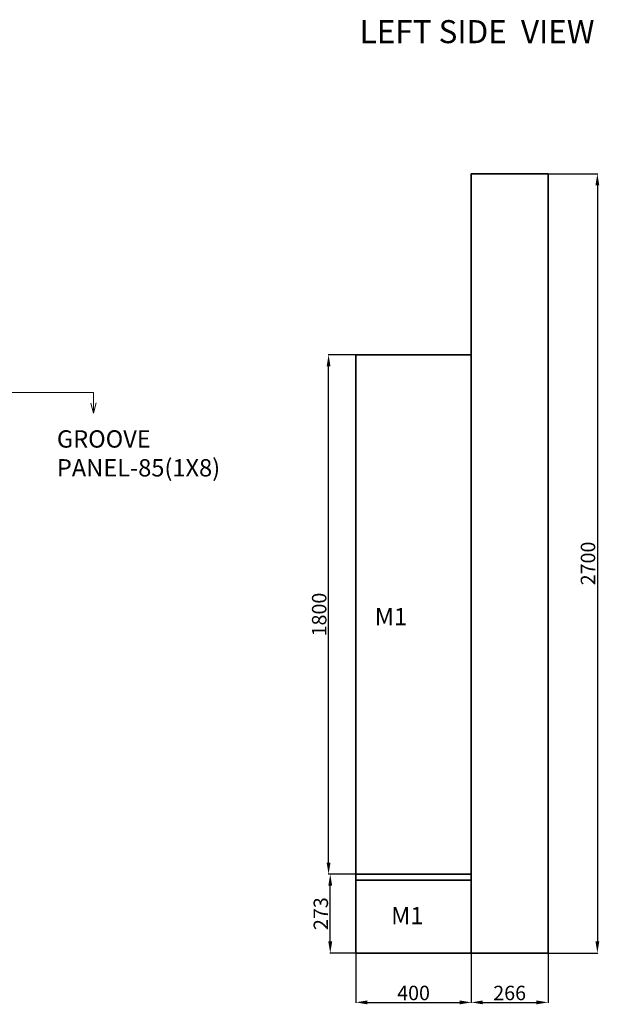
# Model space of a CAD drawing. Units: millimetres. Extents: x 11439 to 24661, y -4767 to -6.
# Tile 5 of 5: x 22652 to 24661, y -4215 to -803. Entities that reach past the tile are written whole.
import ezdxf

# ---------------------------------------------------------------- set-up
doc = ezdxf.new("R2010")
doc.units = ezdxf.units.MM
for name, color, linetype, lineweight in [('A-ANNO-DIMS', 2, 'Continuous', 18), ('A-ANNO-TEXT', 3, 'Continuous', 18), ('A-FURN', 7, 'Continuous', 35)]:
    doc.layers.add(name, color=color, linetype=linetype, lineweight=lineweight)
doc.styles.get("Standard").update_dxf_attribs({"font": 'arial.ttf'})
doc.dimstyles.new('ISO-25', dxfattribs={"dimtxt": 50, "dimasz": 40, "dimexe": 1.25, "dimexo": 0.625, "dimtad": 1, "dimtxsty": 'Standard', "dimcen": 2.5, "dimadec": 0, "dimazin": 0, "dimtfac": 1, "dimtmove": 0, "dimatfit": 3, "dimfxl": 1, "dimarcsym": 0})

# ---------------------------------------------------------------- blocks, each defined once
blk = doc.blocks.new('*D43')
at = {"layer": 'A-ANNO-DIMS', "color": 0, "lineweight": -2, "transparency": 16777216}
for p, q in [((23816.4, -3764.7), (23727.1, -3764.7)), ((23728.3, -3997.7), (23728.3, -3804.7)), ((23816.4, -4037.7), (23727.1, -4037.7))]:
    blk.add_line(p, q, dxfattribs=at)
at = {"layer": 'A-ANNO-DIMS', "color": 0, "transparency": 16777216}
for points in [[(23721.6, -3804.7), (23735, -3804.7), (23728.3, -3764.7)], [(23721.6, -3997.7), (23735, -3997.7), (23728.3, -4037.7)]]:
    blk.add_solid(points, dxfattribs=at)
at = {"layer": 'Defpoints', "color": 0, "transparency": 16777216}
for p in [(23728.3, -3764.7), (23817, -3764.7), (23817, -4037.7)]:
    blk.add_point(p, dxfattribs=at)
at = {"layer": 'A-ANNO-DIMS', "color": 0, "transparency": 16777216, "insert": (23702.1, -3901.2), "char_height": 50, "attachment_point": 5, "rotation": 90}
blk.add_mtext('273', dxfattribs=at)
blk = doc.blocks.new('*D44')
at = {"layer": 'A-ANNO-DIMS', "color": 0, "lineweight": -2, "transparency": 16777216}
for p, q in [((23816.4, -1964.7), (23721.3, -1964.7)), ((23722.5, -3724.7), (23722.5, -2004.7)), ((23816.4, -3764.7), (23721.3, -3764.7))]:
    blk.add_line(p, q, dxfattribs=at)
at = {"layer": 'A-ANNO-DIMS', "color": 0, "transparency": 16777216}
for points in [[(23715.8, -2004.7), (23729.2, -2004.7), (23722.5, -1964.7)], [(23715.8, -3724.7), (23729.2, -3724.7), (23722.5, -3764.7)]]:
    blk.add_solid(points, dxfattribs=at)
at = {"layer": 'Defpoints', "color": 0, "transparency": 16777216}
for p in [(23722.5, -1964.7), (23817, -1964.7), (23817, -3764.7)]:
    blk.add_point(p, dxfattribs=at)
at = {"layer": 'A-ANNO-DIMS', "color": 0, "transparency": 16777216, "insert": (23696.4, -2864.7), "char_height": 50, "attachment_point": 5, "rotation": 90}
blk.add_mtext('1800', dxfattribs=at)
blk = doc.blocks.new('*D54')
at = {"layer": 'A-ANNO-DIMS', "color": 0, "lineweight": -2, "transparency": 16777216}
for p, q in [((23817, -4038.3), (23817, -4209.9)), ((24217, -4038.3), (24217, -4209.9)), ((23857, -4208.7), (24177, -4208.7))]:
    blk.add_line(p, q, dxfattribs=at)
at = {"layer": 'A-ANNO-DIMS', "color": 0, "transparency": 16777216}
for points in [[(23857, -4202), (23857, -4215.4), (23817, -4208.7)], [(24177, -4202), (24177, -4215.4), (24217, -4208.7)]]:
    blk.add_solid(points, dxfattribs=at)
at = {"layer": 'Defpoints', "color": 0, "transparency": 16777216}
for p in [(23817, -4037.7), (24217, -4037.7), (24217, -4208.7)]:
    blk.add_point(p, dxfattribs=at)
at = {"layer": 'A-ANNO-DIMS', "color": 0, "transparency": 16777216, "insert": (24017, -4182.5), "char_height": 50, "attachment_point": 5}
blk.add_mtext('400', dxfattribs=at)
blk = doc.blocks.new('*D55')
at = {"layer": 'A-ANNO-DIMS', "color": 0, "lineweight": -2, "transparency": 16777216}
for p, q in [((24217, -4038.3), (24217, -4209.9)), ((24483, -4038.3), (24483, -4209.9)), ((24257, -4208.7), (24443, -4208.7))]:
    blk.add_line(p, q, dxfattribs=at)
at = {"layer": 'A-ANNO-DIMS', "color": 0, "transparency": 16777216}
for points in [[(24257, -4202), (24257, -4215.4), (24217, -4208.7)], [(24443, -4202), (24443, -4215.4), (24483, -4208.7)]]:
    blk.add_solid(points, dxfattribs=at)
at = {"layer": 'Defpoints', "color": 0, "transparency": 16777216}
for p in [(24217, -4037.7), (24483, -4037.7), (24483, -4208.7)]:
    blk.add_point(p, dxfattribs=at)
at = {"layer": 'A-ANNO-DIMS', "color": 0, "transparency": 16777216, "insert": (24350, -4182.5), "char_height": 50, "attachment_point": 5}
blk.add_mtext('266', dxfattribs=at)
blk = doc.blocks.new('*D56')
at = {"layer": 'A-ANNO-DIMS', "color": 0, "lineweight": -2, "transparency": 16777216}
for p, q in [((24483.6, -1337.7), (24655.3, -1337.7)), ((24654, -1377.7), (24654, -3997.7)), ((24483.6, -4037.7), (24655.3, -4037.7))]:
    blk.add_line(p, q, dxfattribs=at)
at = {"layer": 'A-ANNO-DIMS', "color": 0, "transparency": 16777216}
for points in [[(24647.3, -1377.7), (24660.7, -1377.7), (24654, -1337.7)], [(24647.3, -3997.7), (24660.7, -3997.7), (24654, -4037.7)]]:
    blk.add_solid(points, dxfattribs=at)
at = {"layer": 'Defpoints', "color": 0, "transparency": 16777216}
for p in [(24483, -1337.7), (24483, -4037.7), (24654, -4037.7)]:
    blk.add_point(p, dxfattribs=at)
at = {"layer": 'A-ANNO-DIMS', "color": 0, "transparency": 16777216, "insert": (24627.9, -2687.7), "char_height": 50, "attachment_point": 5, "rotation": 90}
blk.add_mtext('2700', dxfattribs=at)

msp = doc.modelspace()

# ---------------------------------------------------------------- linework, layer by layer
at = {"layer": 'A-ANNO-TEXT'}
for p, q in [((21560.761, -2095.642), (22907.534, -2095.642)), ((22907.534, -2095.642), (22907.534, -2166.511)), ((22907.534, -2166.511), (22898.054, -2132.022)), ((22907.534, -2166.511), (22917.263, -2131.108))]:
    msp.add_line(p, q, dxfattribs=at)
at = {"layer": 'A-FURN'}
for p, q in [((24217.007, -1337.684), (24483.007, -1337.684)), ((24217.007, -1337.684), (24217.007, -4037.684)), ((24483.007, -1337.684), (24483.007, -4037.684)), ((23817.007, -4037.684), (23817.007, -1964.684)), ((23817.007, -1964.684), (24217.007, -1964.684)), ((23817.007, -3764.684), (24217.007, -3764.684)), ((23817.007, -3784.684), (24217.007, -3784.684)), ((23817.007, -4037.684), (24483.007, -4037.684))]:
    msp.add_line(p, q, dxfattribs=at)

# ---------------------------------------------------------------- texts
at = {"layer": 'A-ANNO-TEXT', "attachment_point": 1}
for s, insert, char_height in [('LEFT SIDE  VIEW', (23830.171, -804.835), 80), ('GROOVE \\PPANEL-85(1X8)', (22780.973, -2226.26), 60), ('\\P    M1', (23809.23, -2741.895), 60), ('\\P    M1', (23865.925, -3777.968), 60)]:
    msp.add_mtext_dynamic_manual_height_columns(s, width=1074.7282, gutter_width=12.5, heights=[0], dxfattribs=dict(at, insert=insert, char_height=char_height))

# ---------------------------------------------------------------- dimensions: what is measured, and where the dimension line sits
at = {"layer": 'A-ANNO-DIMS'}
for base, p1, p2, override, picture, middle in [((24654.007, -4037.684), (24483.007, -1337.684), (24483.007, -4037.684), {"dimdec": 0, "dimlfac": 1, "dimrnd": 0, "dimzin": 0, "dimdsep": 46, "dimlunit": 2}, '*D56', (24627.853, -2687.684)), ((23722.514, -1964.684), (23817.007, -3764.684), (23817.007, -1964.684), {"dimclrd": 0, "dimclre": 0, "dimclrt": 0}, '*D44', (23696.36, -2864.684)), ((23728.303, -3764.684), (23817.007, -4037.684), (23817.007, -3764.684), {"dimclrd": 0, "dimclre": 0, "dimclrt": 0}, '*D43', (23702.133, -3901.184))]:
    dim = msp.add_linear_dim(base=base, p1=p1, p2=p2, angle=90, dimstyle='ISO-25', override=override, dxfattribs=at)
    dim.commit()
    dim.dimension.update_dxf_attribs({"geometry": picture, "text_midpoint": middle})
for base, p1, p2, picture, middle in [((24217.007, -4208.684), (23817.007, -4037.684), (24217.007, -4037.684), '*D54', (24017.007, -4182.531)), ((24483.007, -4208.684), (24217.007, -4037.684), (24483.007, -4037.684), '*D55', (24350.007, -4182.531))]:
    dim = msp.add_linear_dim(base=base, p1=p1, p2=p2, dimstyle='ISO-25', override={"dimdec": 0, "dimlfac": 1, "dimrnd": 0, "dimzin": 0, "dimdsep": 46, "dimlunit": 2}, dxfattribs=at)
    dim.commit()
    dim.dimension.update_dxf_attribs({"geometry": picture, "text_midpoint": middle})

doc.saveas('drawing.dxf')
